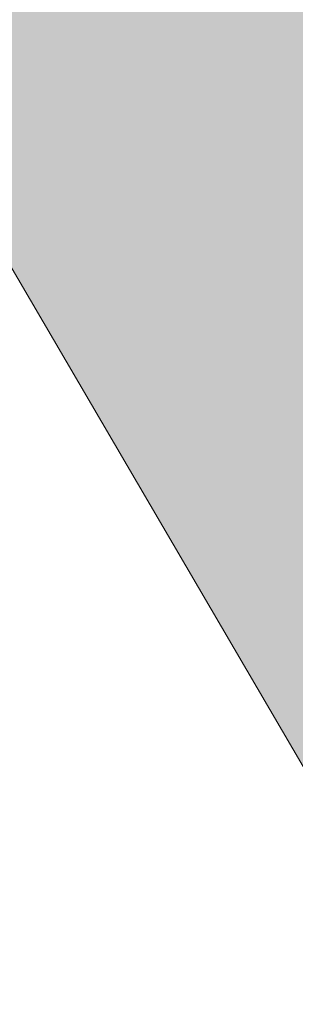
# Model space of a CAD drawing. Units: inches. Extents: x 2091 to 2899, y 967 to 2217.
# Tile 242 of 256: x 2213.361 to 2214.578, y 1131.245 to 1135.592. Entities that reach past the tile are written whole.
import ezdxf

# ---------------------------------------------------------------- set-up
doc = ezdxf.new("R2010")
doc.units = ezdxf.units.IN
doc.layers.add('A-WALL-PATT', color=141, linetype='Continuous', lineweight=13, true_color=0xadddf7)
doc.layers.add('L-PLNT-PATT', color=114, linetype='Continuous', lineweight=13, true_color=0x139b48)
doc.layers.add('L-PLNT-TREE', color=94, linetype='Continuous', lineweight=13)

# ---------------------------------------------------------------- blocks, each defined once
blk = doc.blocks.new('*U25')
blk.add_lwpolyline([(-1139.42368, 1783.79628), (-1216.11644, 1685.47796), (-1117.5111, 1601.2033), (-1051.7759, 1643.3419), (-1126.09884, 1521.20092), (-1072.10606, 1527.49758), (-1079.90386, 1416.93646), (-1259.93906, 1179.83508), (-1479.05978, 1165.78888), (-1577.66258, 1109.60662), (-1742.00312, 927.01364), (-1676.26538, 814.64658), (-1270.89408, 828.69278), (-1194.20386, 772.51052), (-1007.95074, 856.78518), (-876.4778, 575.87134), (-821.70016, 575.87134), (-569.71184, 884.87504)])

msp = doc.modelspace()

# ---------------------------------------------------------------- hatches: boundary and pattern name
at = {"layer": 'A-WALL-PATT'}
h = msp.add_hatch(color=256, dxfattribs=at)
h.dxf.hatch_style = 1
h.paths.add_polyline_path([(2803.1436, 2050.9191), (2203.1436, 2050.9191), (2203.1436, 1090.9191), (2803.1436, 1090.9191)])
h.paths.add_polyline_path([(2635.7989, 1147.5405), (2674.5241, 1147.5405, 0.376086), (2678.5297, 1152.8802), (2678.5297, 1159.5565, 0.333335), (2674.5243, 1163.5618), (2674.5243, 1163.5619), (2674.5243, 1192.9344), (2635.806, 1192.9344), (2597.0876, 1192.9344), (2597.0876, 1163.5618, 0.333335), (2593.0823, 1159.5565), (2593.0823, 1152.8802, 0.376086), (2597.0879, 1147.5405)], flags=0)
h.paths.add_polyline_path([(2436.0104, 1278.2408, 0.000483), (2435.9526, 1278.215, -0.001328), (2435.9356, 1278.1117, -0.001711), (2436.1164, 1278.0408, 0.002185)], flags=0)
h.paths.add_polyline_path([(2794.1436, 1143.4191), (2794.1436, 1347.4191), (2543.3702, 1347.4191), (2543.3702, 1351.9191), (2794.1436, 1351.9191), (2794.1436, 1392.7136), (2793.9474, 1392.7136), (2793.9474, 1473.5369), (2794.1436, 1473.5369), (2794.1436, 1531.9191), (2650.1436, 1531.9191), (2650.1436, 1536.4191), (2794.1436, 1536.4191), (2794.1436, 1692.4191), (2609.3756, 1692.4191), (2609.3756, 1644.4191), (2604.8756, 1644.4191), (2604.8756, 1744.9191), (2609.3756, 1744.9191), (2609.3756, 1696.9191), (2794.1436, 1696.9191), (2794.1436, 1780.9191), (2609.6436, 1780.9191), (2493.8756, 1780.9191), (2493.8756, 1785.4191), (2609.6436, 1785.4191), (2794.1436, 1785.4191), (2794.1436, 1847.9388), (2793.9512, 1847.9388), (2793.9512, 1928.7622), (2794.1436, 1928.7622), (2794.1436, 1941.4191), (2614.1436, 1941.4191), (2614.1436, 1821.4191), (2609.6436, 1821.4191), (2609.6436, 1941.4191), (2392.1436, 1941.4191), (2392.1436, 1819.9191), (2387.6436, 1819.9191), (2387.6436, 1941.4191), (2212.1436, 1941.4191), (2212.1436, 1783.9191), (2392.1436, 1783.9191), (2392.1436, 1780.9191), (2212.1436, 1780.9191), (2212.1436, 1629.4191), (2387.6436, 1629.4191), (2387.6436, 1744.9191), (2392.1436, 1744.9191), (2392.1436, 1627.9191), (2317.1436, 1627.9191), (2317.1436, 1551.4191), (2317.1436, 1536.4191), (2459.3836, 1536.4191), (2459.3836, 1602.3965), (2463.8836, 1602.3965), (2463.8836, 1531.9191), (2456.6436, 1531.9191), (2456.6436, 1529.9191), (2452.1436, 1529.9191), (2452.1436, 1531.9191), (2312.6436, 1531.9191), (2312.6436, 1551.4191), (2306.1436, 1551.4191), (2306.1436, 1555.9191), (2308.1436, 1555.9191), (2308.1436, 1551.4191), (2312.6436, 1551.4191), (2312.6436, 1627.9191), (2212.1436, 1627.9191), (2212.1436, 1555.9191), (2270.1436, 1555.9191), (2270.1436, 1551.4191), (2212.1436, 1551.4191), (2212.1436, 1351.9191), (2272.1436, 1351.9191), (2272.1436, 1347.4191), (2212.1436, 1347.4191), (2212.1436, 1275.4191), (2308.1436, 1275.4191), (2308.1436, 1351.9191), (2452.1436, 1351.9191), (2452.1436, 1493.9191), (2456.6436, 1493.9191), (2456.6436, 1347.4191), (2312.6436, 1347.4191), (2312.6436, 1270.9191), (2212.1436, 1270.9191), (2212.1436, 1099.9191), (2281.2375, 1099.9191), (2282.871, 1110.9138), (2282.0083, 1116.9966), (2278.5577, 1121.4204), (2268.2056, 1128.0562), (2272.0876, 1128.0562), (2273.8129, 1131.927), (2279.4203, 1134.6919), (2285.0278, 1135.2449), (2287.6158, 1137.4568), (2288.0471, 1138.0098), (2289.3411, 1140.7747), (2291.0665, 1139.6687), (2292.3605, 1135.2449), (2295.3798, 1136.9038), (2296.2425, 1135.7979), (2297.1052, 1133.033), (2300.1246, 1138.0098), (2303.1439, 1138.0098), (2304.4379, 1135.7979), (2303.1439, 1133.586), (2306.5946, 1134.6919), (2307.8887, 1133.033), (2310.908, 1135.2449), (2313.9274, 1134.1389), (2315.6269, 1132.4271), (2308.32, 1117.5496), (2290.2038, 1109.8079), (2288.9098, 1103.1721), (2289.2723, 1099.9191), (2434.9182, 1099.9191), (2431.5932, 1124.7881), (2429.9302, 1169.5531), (2430.9272, 1240.5197), (2435.6589, 1238.1861), (2437.1352, 1196.5541), (2438.7982, 1143.9731), (2442.6782, 1111.9981), (2446.5582, 1099.9191), (2794.1436, 1099.9191), (2794.1436, 1138.9191), (2548.0324, 1138.9191), (2548.0324, 1143.4191), (2548.0324, 1148.8191), (2546.6685, 1148.0316), (2528.6857, 1179.1786, 0.256256), (2512.0324, 1148.8191), (2512.0324, 1143.4191), (2512.0324, 1138.9191), (2507.5324, 1138.9191), (2507.5324, 1143.4191), (2507.5324, 1148.8191, 0.256256), (2490.8792, 1179.1786), (2472.8964, 1148.0316), (2471.5324, 1148.8191), (2471.5324, 1143.4191), (2467.0324, 1143.4191), (2467.0324, 1269.9458, 0.039061), (2460.91, 1273.5801), (2467.0324, 1273.5801), (2467.0324, 1286.3254, 0.014511), (2465.2162, 1286.7619), (2467.0324, 1287.0526), (2467.0324, 1323.4191), (2471.5324, 1323.4191), (2471.5324, 1148.8191), (2489.5324, 1179.996), (2490.8964, 1179.2085), (2490.8792, 1179.1786, -0.256256), (2507.5324, 1148.8191), (2507.5324, 1143.4191), (2512.0324, 1143.4191), (2512.0324, 1148.8191, -0.256256), (2528.6857, 1179.1786), (2528.6685, 1179.2085), (2530.0324, 1179.996), (2548.0324, 1148.8191), (2548.0324, 1143.4191)], flags=16)
h.paths.add_polyline_path([(2607.7685, 1200.9451), (2607.7685, 1265.0306), (2597.0876, 1281.052), (2619.7846, 1281.052), (2627.7953, 1337.1269), (2635.7989, 1337.1269), (2643.8167, 1337.1269), (2651.8274, 1281.052), (2674.5243, 1281.052), (2663.8434, 1265.0306), (2663.8434, 1200.9451), (2635.806, 1200.9451)], flags=0)
edge = h.paths.add_edge_path(flags=0)
edge.add_ellipse((13303.8962, 1272.9987), major_axis=(-10595.313, 0), ratio=0.8423038701, start_angle=0.62823722, end_angle=0.6465541, ccw=False)
edge.add_ellipse((2711.7004, 1156.8527), major_axis=(2.2198, 0), ratio=0.842304, start_angle=111.5352, end_angle=180.6282, ccw=False)
edge.add_ellipse((13303.1563, 1272.9987), major_axis=(-10593.0263, 0), ratio=0.8423038695, start_angle=0.52827147, end_angle=0.6465541, ccw=False)
edge.add_line((2710.7646, 1175.3333), (2710.13, 1175.3333))
edge.add_ellipse((2710.13, 1176.5798), major_axis=(1.4798, 0), ratio=0.842304, start_angle=180, end_angle=270, ccw=False)
edge.add_line((2708.6501, 1176.5798), (2708.6501, 1200.7829))
edge.add_ellipse((2710.13, 1200.7829), major_axis=(1.4798, 0), ratio=0.842304, start_angle=90, end_angle=180, ccw=False)
edge.add_line((2710.13, 1202.0294), (2710.4651, 1202.0294))
edge.add_ellipse((13303.1563, 1272.9987), major_axis=(-10593.0263, 0), ratio=0.8423038695, start_angle=-0.09022909, end_angle=0.38386678, ccw=False)
edge.add_ellipse((2710.13, 1290.927), major_axis=(-1.4798, 0), ratio=0.842304, start_angle=0, end_angle=90, ccw=False)
edge.add_line((2708.6501, 1290.927), (2708.6501, 1315.1302))
edge.add_ellipse((2710.13, 1315.1302), major_axis=(-1.4798, 0), ratio=0.842304, start_angle=-90, end_angle=0, ccw=False)
edge.add_line((2710.13, 1316.3767), (2710.7063, 1316.3767))
edge.add_ellipse((3238.4017, 1296.2896), major_axis=(528.234, 0), ratio=0.84230387, start_angle=176.349572, end_angle=177.82005, ccw=False)
edge.add_ellipse((2775.063, 1071.4507), major_axis=(313.3078, 0), ratio=0.84230387, start_angle=102.125966, end_angle=103.780529, ccw=False)
edge.add_ellipse((2775.063, 1078.3057), major_axis=(-305.3029, 0), ratio=0.84230387, start_angle=-79.790461, end_angle=-77.555373, ccw=False)
edge.add_ellipse((2695.1418, 1541.9754), major_axis=(-250.9602, 0), ratio=0.84230387, start_angle=99.256566, end_angle=102.554933)
edge.add_line((2741.4103, 1334.2143), (2747.1325, 1337.3785))
edge.add_ellipse((2747.5386, 1336.8575), major_axis=(-0.7399, 0), ratio=0.842304, start_angle=270, end_angle=307.9331, ccw=False)
edge.add_ellipse((2747.5386, 1336.8575), major_axis=(-0.7399, 0), ratio=0.842304, start_angle=232.0669, end_angle=270, ccw=False)
edge.add_line((2747.9447, 1337.3785), (2753.6669, 1334.2143))
edge.add_ellipse((2799.9355, 1541.9754), major_axis=(250.9602, 0), ratio=0.84230387, start_angle=257.445067, end_angle=260.743434)
edge.add_ellipse((2720.0142, 1078.3057), major_axis=(305.3029, 0), ratio=0.84230387, start_angle=77.555373, end_angle=79.790461, ccw=False)
edge.add_ellipse((2720.0142, 1071.4507), major_axis=(-313.3078, 0), ratio=0.84230387, start_angle=256.219471, end_angle=257.874034, ccw=False)
edge.add_ellipse((2256.6755, 1296.2896), major_axis=(-528.234, 0), ratio=0.84230387, start_angle=182.17995, end_angle=183.650428, ccw=False)
edge.add_line((2784.3709, 1316.3767), (2784.9472, 1316.3767))
edge.add_ellipse((2784.9472, 1315.1302), major_axis=(1.4798, 0), ratio=0.842304, start_angle=0, end_angle=90, ccw=False)
edge.add_line((2786.4271, 1315.1302), (2786.4271, 1290.927))
edge.add_ellipse((2784.9472, 1290.927), major_axis=(1.4798, 0), ratio=0.842304, start_angle=270, end_angle=360, ccw=False)
edge.add_ellipse((-7808.0791, 1272.9987), major_axis=(10593.0263, 0), ratio=0.8423038695, start_angle=-0.38386678, end_angle=0.09022909, ccw=False)
edge.add_line((2784.6122, 1202.0294), (2784.9472, 1202.0294))
edge.add_ellipse((2784.9472, 1200.7829), major_axis=(1.4798, 0), ratio=0.842304, start_angle=0, end_angle=90, ccw=False)
edge.add_line((2786.4271, 1200.7829), (2786.4271, 1176.5798))
edge.add_ellipse((2784.9472, 1176.5798), major_axis=(-1.4798, 0), ratio=0.842304, start_angle=90, end_angle=180, ccw=False)
edge.add_line((2784.9472, 1175.3333), (2784.3126, 1175.3333))
edge.add_ellipse((-7808.0791, 1272.9987), major_axis=(10593.0263, 0), ratio=0.8423038695, start_angle=-0.6186432, end_angle=-0.52827147, ccw=False)
edge.add_ellipse((2783.3768, 1156.8527), major_axis=(-2.2198, 0), ratio=0.842304, start_angle=179.3718, end_angle=248.4648, ccw=False)
edge.add_ellipse((-7808.819, 1272.9987), major_axis=(-10595.313, 0), ratio=0.8423038658, start_angle=179.35344592, end_angle=179.3717628, ccw=False)
edge.add_ellipse((2780.2973, 1153.5008), major_axis=(-5.2464, 0), ratio=0.842304, start_angle=90, end_angle=179.3534, ccw=False)
edge.add_line((2780.2973, 1149.0817), (2714.7799, 1149.0817))
edge.add_ellipse((2714.7799, 1153.5008), major_axis=(5.2464, 0), ratio=0.842304, start_angle=180.6466, end_angle=270, ccw=False)
edge = h.paths.add_edge_path(flags=0)
edge.add_line((2718.1874, 1151.0078), (2718.1874, 1170.4724))
edge.add_ellipse((2721.1471, 1170.4724), major_axis=(-2.9597, 0), ratio=0.842304, start_angle=-90, end_angle=0, ccw=False)
edge.add_line((2721.1471, 1172.9653), (2773.9302, 1172.9653))
edge.add_ellipse((2773.9302, 1170.4724), major_axis=(-2.9597, 0), ratio=0.842304, start_angle=180, end_angle=270, ccw=False)
edge.add_line((2776.8899, 1170.4724), (2776.8899, 1151.0078))
edge.add_line((2776.8899, 1151.0078), (2718.1874, 1151.0078))
edge = h.paths.add_edge_path(flags=0)
edge.add_line((2718.1874, 1180.2342), (2718.1874, 1199.0578))
edge.add_ellipse((2747.5386, 1320.3986), major_axis=(147.0179, 0), ratio=0.84230387, start_angle=256.401865, end_angle=283.598135)
edge.add_line((2776.8899, 1199.0578), (2776.8899, 1180.2342))
edge.add_ellipse((2747.5386, 1301.575), major_axis=(147.0179, 0), ratio=0.84230387, start_angle=256.401865, end_angle=283.598135, ccw=False)
edge = h.paths.add_edge_path(flags=0)
edge.add_ellipse((13303.1563, 1272.9987), major_axis=(-10591.5465, 0), ratio=0.8423038696, start_angle=0.05559431, end_angle=0.37776419, ccw=False)
edge.add_line((2711.6169, 1262.7217), (2715.6674, 1249.4954))
edge.add_ellipse((6413.892, 1241.6919), major_axis=(-3698.2362, 0), ratio=0.84230387, start_angle=-0.1208974, end_angle=0.3640763)
edge.add_line((2715.761, 1218.1925), (2711.9343, 1203.1674))
edge = h.paths.add_edge_path(flags=0)
edge.add_line((2718.1874, 1251.0746), (2716.0025, 1267.4504))
edge.add_ellipse((2742.1512, 1202.1895), major_axis=(81.7726, 0), ratio=0.8423039, start_angle=94.277421, end_angle=111.834954, ccw=False)
edge.add_line((2737.0097, 1270.9306), (2758.0675, 1270.9306))
edge.add_ellipse((2752.9261, 1202.1895), major_axis=(81.7726, 0), ratio=0.8423039, start_angle=68.165046, end_angle=85.722579, ccw=False)
edge.add_line((2779.0747, 1267.4504), (2776.8899, 1251.0746))
edge.add_ellipse((2750.3381, 1187.8854), major_axis=(79.5797, 0), ratio=0.8423039, start_angle=67.208085, end_angle=85.12993)
edge.add_line((2756.0347, 1254.7437), (2739.0426, 1254.7437))
edge.add_ellipse((2744.7392, 1187.8854), major_axis=(79.5797, 0), ratio=0.8423039, start_angle=94.87007, end_angle=112.791915)
edge = h.paths.add_edge_path(flags=0)
edge.add_line((2783.1429, 1203.1674), (2779.3162, 1218.1925))
edge.add_ellipse((-918.8147, 1241.6919), major_axis=(3698.2362, 0), ratio=0.84230387, start_angle=-0.3640763, end_angle=0.1208974)
edge.add_line((2779.4098, 1249.4954), (2783.4604, 1262.7217))
edge.add_ellipse((-7808.0791, 1272.9987), major_axis=(-10591.5465, 0), ratio=0.8423038695, start_angle=179.62223581, end_angle=179.94440569, ccw=False)
edge = h.paths.add_edge_path(flags=0)
edge.add_ellipse((2734.2009, 1286.6904), major_axis=(-0.3566, 6.3401), ratio=0.603834, start_angle=89.00201, end_angle=253.65741, ccw=False)
edge.add_line((2730.369, 1286.5418), (2730.369, 1301.352))
edge.add_line((2730.369, 1301.352), (2735.9133, 1305.2148))
edge.add_ellipse((2736.3849, 1304.7346), major_axis=(0.7399, 0), ratio=0.842304, start_angle=90, end_angle=134.4802, ccw=False)
edge.add_line((2736.3849, 1305.3578), (2738.0328, 1305.3578))
edge.add_line((2738.0328, 1305.3578), (2738.0328, 1307.7079))
edge.add_ellipse((2794.2016, 1307.7079), major_axis=(56.1689, 0), ratio=0.8423039, start_angle=150.56143, end_angle=180, ccw=False)
edge.add_ellipse((2700.8756, 1307.7079), major_axis=(-56.1689, 0), ratio=0.8423039, start_angle=180, end_angle=209.43857, ccw=False)
edge.add_line((2757.0444, 1307.7079), (2757.0444, 1305.3578))
edge.add_line((2757.0444, 1305.3578), (2758.6923, 1305.3578))
edge.add_ellipse((2758.6923, 1304.7346), major_axis=(-0.7399, 0), ratio=0.842304, start_angle=225.5198, end_angle=270, ccw=False)
edge.add_line((2759.1639, 1305.2148), (2764.7082, 1301.352))
edge.add_line((2764.7082, 1301.352), (2764.7082, 1286.5418))
edge.add_ellipse((2760.8763, 1286.6904), major_axis=(0.3566, 6.3401), ratio=0.603834, start_angle=106.34259, end_angle=270.99799, ccw=False)
edge.add_line((2757.0444, 1285.7971), (2757.0444, 1307.7079))
edge.add_ellipse((2700.8756, 1307.7079), major_axis=(-56.1689, 0), ratio=0.8423039, start_angle=180, end_angle=209.43857)
edge.add_ellipse((2794.2016, 1307.7079), major_axis=(56.1689, 0), ratio=0.8423039, start_angle=150.56143, end_angle=180)
edge.add_line((2738.0328, 1307.7079), (2738.0328, 1285.7971))
h.paths.add_polyline_path([(2417.8123, 1104.4497), (2413.4923, 1102.5297), (2410.6123, 1103.9697), (2409.1723, 1106.3697), (2407.2523, 1107.3297), (2406.2923, 1109.7297), (2405.3323, 1114.0497), (2405.3323, 1117.8897), (2406.2923, 1120.1297), (2407.2523, 1119.8097), (2408.8483, 1118.3277), (2410.1739, 1119.4242), (2410.2113, 1120.4057), (2411.0407, 1121.4191), (2410.6993, 1119.8587), (2410.1739, 1119.4242), (2410.0885, 1117.1761), (2411.1328, 1116.2063), (2413.9723, 1119.3297), (2416.8523, 1120.7697), (2416.8697, 1120.7988), (2417.0351, 1119.4051), (2417.8962, 1118.1434), (2418.2923, 1118.3697), (2419.5444, 1120.0393), (2419.3609, 1118.3875), (2419.0321, 1119.3562), (2418.3989, 1118.5119), (2419.2523, 1114.5297), (2418.7941, 1107.1988)], flags=0)
h.paths.add_polyline_path([(2508.8702, 1347.4191), (2508.3702, 1347.4191), (2508.3702, 1351.9191), (2508.8702, 1351.9191)], flags=0)
h.paths.add_polyline_path([(2473.3702, 1347.4191), (2472.3702, 1347.4191), (2467.8702, 1347.4191), (2467.8702, 1455.4191), (2472.3702, 1455.4191), (2472.3702, 1352.4191), (2473.3702, 1352.4191)], flags=0)
h.paths.add_polyline_path([(2352.1062, 1217.4462), (2349.2262, 1218.8862), (2347.7862, 1221.2862), (2345.8662, 1222.2462), (2344.9062, 1224.6462), (2343.9462, 1228.9662), (2343.9462, 1232.8062), (2344.9062, 1235.0462), (2345.8662, 1234.7262), (2347.4623, 1233.2442), (2348.7879, 1234.3407), (2348.8252, 1235.3222), (2349.6547, 1236.3355), (2349.3132, 1234.7752), (2348.7879, 1234.3407), (2348.7024, 1232.0926), (2349.7468, 1231.1228), (2352.5862, 1234.2462), (2355.4662, 1235.6862), (2355.4837, 1235.7153), (2355.649, 1234.3216), (2356.5102, 1233.0599), (2356.9062, 1233.2862), (2358.1584, 1234.9558), (2357.9749, 1233.304), (2357.6461, 1234.2726), (2357.0129, 1233.4284), (2357.8662, 1229.4462), (2357.4081, 1222.1153), (2356.4262, 1219.3662)], flags=0)
h.paths.add_polyline_path([(2348.2968, 1112.2244), (2347.0138, 1112.3104), (2345.5298, 1114.1274), (2345.7318, 1115.8584), (2346.8118, 1116.9824), (2346.8118, 1114.6464), (2345.8668, 1114.2144), (2346.8798, 1114.3004)], flags=0)
h.paths.add_polyline_path([(2347.0138, 1110.9264), (2346.2718, 1110.4934), (2346.6098, 1111.1864)], flags=0)
h.paths.add_polyline_path([(2345.8668, 1118.1944), (2345.5298, 1117.3294), (2343.7078, 1118.0214), (2344.3828, 1118.6264)], flags=0)
h.paths.add_polyline_path([(2346.6768, 1109.2824), (2346.0698, 1108.0714), (2345.8668, 1110.0614)], flags=0)
h.paths.add_polyline_path([(2345.0568, 1119.7514), (2343.6398, 1119.7514), (2343.9778, 1121.1354)], flags=0)
h.paths.add_polyline_path([(2345.2598, 1116.5504), (2345.1248, 1115.8584), (2344.9218, 1115.6854), (2344.7198, 1116.3774)], flags=0)
h.paths.add_polyline_path([(2345.6648, 1112.3104), (2345.4618, 1111.5324), (2344.0448, 1111.9644), (2344.6518, 1112.5704)], flags=0)
h.paths.add_polyline_path([(2345.1918, 1113.3494), (2344.4498, 1113.8684), (2344.7198, 1114.3874)], flags=0)
h.paths.add_polyline_path([(2344.6518, 1116.8094), (2344.1798, 1115.6854), (2344.6518, 1115.3394), (2343.9098, 1114.9064), (2343.0328, 1115.9444), (2343.6398, 1116.4634)], flags=0)
h.paths.add_polyline_path([(2345.8668, 1106.6864), (2344.9898, 1105.5624), (2344.5168, 1106.6004)], flags=0)
h.paths.add_polyline_path([(2344.8548, 1110.0614), (2344.5168, 1109.2824), (2344.1128, 1109.7154)], flags=0)
h.paths.add_polyline_path([(2344.0448, 1113.5224), (2343.4378, 1113.0894), (2342.7628, 1113.9544)], flags=0)
h.paths.add_polyline_path([(2344.3148, 1111.0124), (2342.9648, 1110.3204), (2342.9648, 1111.0994)], flags=0)
h.paths.add_polyline_path([(2345.1248, 1104.6974), (2344.5848, 1103.7454), (2344.4498, 1104.2644)], flags=0)
h.paths.add_polyline_path([(2342.8298, 1121.2224), (2341.7498, 1120.5304), (2340.5358, 1121.0494), (2340.1308, 1121.8284), (2340.6708, 1122.9524), (2341.1428, 1121.8284), (2341.6148, 1122.0014)], flags=0)
h.paths.add_polyline_path([(2342.9648, 1119.7514), (2343.0328, 1118.4534), (2342.0878, 1118.0214), (2342.0198, 1119.4914)], flags=0)
h.paths.add_polyline_path([(2342.6948, 1116.8964), (2341.9528, 1116.6364), (2342.0198, 1117.3294)], flags=0)
h.paths.add_polyline_path([(2343.0328, 1112.2244), (2342.0198, 1111.7914), (2341.5478, 1112.2244), (2342.3578, 1113.3494)], flags=0)
h.paths.add_polyline_path([(2343.7748, 1104.4374), (2342.6278, 1102.8804), (2342.6948, 1104.6104), (2343.4378, 1105.1294)], flags=0)
h.paths.add_polyline_path([(2342.0198, 1115.0794), (2340.8058, 1115.5124), (2340.9408, 1116.3774)], flags=0)
h.paths.add_polyline_path([(2341.4808, 1120.0974), (2341.4808, 1119.4054), (2341.0758, 1119.5784), (2341.1428, 1120.0974)], flags=0)
h.paths.add_polyline_path([(2341.8178, 1114.4734), (2340.9408, 1113.0894), (2340.8058, 1114.5604)], flags=0)
h.paths.add_polyline_path([(2341.1428, 1118.5404), (2340.9408, 1116.9824), (2339.0508, 1117.6754), (2339.0508, 1118.6264)], flags=0)
h.paths.add_polyline_path([(2342.6948, 1101.6684), (2341.9528, 1101.8414), (2342.5598, 1102.3614)], flags=0)
h.paths.add_polyline_path([(2340.3328, 1119.6654), (2338.4438, 1119.5784), (2337.9038, 1120.3574), (2339.6578, 1120.6164)], flags=0)
h.paths.add_polyline_path([(2340.3328, 1115.3394), (2340.0628, 1113.6954), (2339.3878, 1115.3394)], flags=0)
h.paths.add_polyline_path([(2341.8178, 1103.8314), (2341.5478, 1102.8804), (2341.1428, 1103.6584)], flags=0)
h.paths.add_polyline_path([(2339.0508, 1122.8664), (2337.2958, 1121.8284), (2337.0938, 1123.1254), (2337.7688, 1123.8184)], flags=0)
h.paths.add_polyline_path([(2339.1178, 1121.7414), (2338.8478, 1121.2224), (2338.1738, 1121.0494), (2338.3758, 1121.5684)], flags=0)
h.paths.add_polyline_path([(2339.1858, 1119.3194), (2338.6458, 1118.7134), (2338.2408, 1118.1074), (2338.2408, 1118.8864)], flags=0)
h.paths.add_polyline_path([(2341.1428, 1101.9284), (2340.6028, 1101.2364), (2340.0628, 1101.8414), (2340.6028, 1102.3614)], flags=0)
h.paths.add_polyline_path([(2337.6338, 1117.7614), (2336.6208, 1118.2804), (2337.2958, 1118.9724)], flags=0)
h.paths.add_polyline_path([(2336.8238, 1119.5784), (2334.7988, 1118.9724), (2335.2038, 1120.3574), (2336.5538, 1120.8764)], flags=0)
h.paths.add_polyline_path([(2339.1178, 1100.4574), (2337.3638, 1100.5434), (2336.7558, 1101.2364)], flags=0)
h.paths.add_polyline_path([(2336.3508, 1122.4334), (2336.0138, 1121.9144), (2334.9338, 1122.4334), (2334.5288, 1123.4714), (2335.7438, 1122.7794)], flags=0)
h.paths.add_polyline_path([(2334.7318, 1120.8764), (2334.2588, 1120.3574), (2334.0568, 1120.7894), (2334.5968, 1121.3084)], flags=0)
h.paths.add_polyline_path([(2334.4618, 1122.1744), (2332.5718, 1121.3084), (2331.3568, 1122.1744), (2332.0998, 1122.8664)], flags=0)
h.paths.add_polyline_path([(2334.2588, 1118.5404), (2333.3818, 1118.4534), (2333.6518, 1119.3194)], flags=0)
h.paths.add_polyline_path([(2335.5418, 1102.2744), (2334.1918, 1102.6204), (2335.2718, 1103.3124)], flags=0)
h.paths.add_polyline_path([(2332.7068, 1119.6654), (2331.6948, 1120.4434), (2332.5048, 1120.7894)], flags=0)
h.paths.add_polyline_path([(2334.7318, 1101.1494), (2333.5168, 1101.5824), (2333.9888, 1101.7554)], flags=0)
h.paths.add_polyline_path([(2332.6398, 1116.6364), (2331.0868, 1116.2904), (2331.9648, 1118.1944)], flags=0)
h.paths.add_polyline_path([(2330.7498, 1121.5684), (2330.2768, 1120.2704), (2328.5228, 1119.3194), (2328.9948, 1121.0494)], flags=0)
h.paths.add_polyline_path([(2330.7498, 1118.6264), (2330.0078, 1117.5024), (2329.8728, 1118.0214)], flags=0)
h.paths.add_polyline_path([(2332.0998, 1102.3614), (2330.5468, 1102.0144), (2331.6948, 1102.9664)], flags=0)
h.paths.add_polyline_path([(2329.5348, 1113.6084), (2329.0628, 1112.3104), (2328.5898, 1113.3494)], flags=0)
h.paths.add_polyline_path([(2328.3878, 1117.8484), (2327.5098, 1116.5504), (2327.1728, 1117.7614)], flags=0)
h.paths.add_polyline_path([(2329.7378, 1106.5134), (2329.5348, 1105.3024), (2328.2528, 1106.0814)], flags=0)
h.paths.add_polyline_path([(2328.6578, 1114.3874), (2328.0498, 1114.1274), (2328.3198, 1114.9064)], flags=0)
h.paths.add_polyline_path([(2328.3198, 1112.2244), (2327.1058, 1112.1374), (2326.7008, 1112.6564)], flags=0)
h.paths.add_polyline_path([(2326.9028, 1115.2524), (2326.7008, 1114.1274), (2325.2158, 1113.6084), (2326.0928, 1115.3394)], flags=0)
h.paths.add_polyline_path([(2326.6328, 1108.3304), (2326.0928, 1107.3794), (2325.8908, 1108.5034), (2326.4978, 1109.1094)], flags=0)
h.paths.add_polyline_path([(2615.1436, 1531.9191), (2609.6436, 1531.9191), (2609.6436, 1620.4191), (2614.1436, 1620.4191), (2614.1436, 1536.4191), (2615.1436, 1536.4191)], flags=0)
h.paths.add_polyline_path([(2545.1436, 1563.4191), (2464.1436, 1563.4191), (2464.1436, 1632.4191), (2509.1436, 1632.4191), (2509.1436, 1627.9191), (2509.1436, 1603.9191), (2468.6436, 1603.9191), (2468.6436, 1567.9191), (2540.6436, 1567.9191), (2540.6436, 1591.9191), (2545.1436, 1591.9191)], flags=0)
h.paths.add_polyline_path([(2388.969, 1549.9857), (2357.4342, 1549.9857), (2357.4342, 1623.3608), (2399.3628, 1623.3608), (2435.6895, 1623.3608), (2435.5925, 1602.5593), (2435.5925, 1602.3965), (2388.969, 1602.3965)], flags=0)
h.paths.add_polyline_path([(2388.8806, 1555.8092), (2374.9044, 1555.8092), (2374.9044, 1600.5716), (2374.9044, 1615.4576), (2406.3509, 1615.4576), (2406.3509, 1618.9394), (2412.1743, 1615.4576), (2406.3509, 1611.9759), (2406.3509, 1615.4576), (2388.8806, 1615.4576)], flags=0)
h.paths.add_polyline_path([(2568.8756, 1644.4191), (2453.3756, 1644.4191), (2453.3756, 1785.4191), (2457.8756, 1785.4191), (2457.8756, 1648.9191), (2568.8756, 1648.9191)], flags=0)
h.paths.add_polyline_path([(2212.1436, 1945.9191), (2212.1436, 2041.9191), (2794.1436, 2041.9191), (2794.1436, 1945.9191)], flags=16)
h.paths.add_polyline_path([(2271.0827, 1964.3172), (2776.853, 1964.3172), (2776.853, 2037.1696), (2271.0827, 2037.1696)], flags=8)
h.paths.add_polyline_path([(2380.6493, 1536.8241), (2461.0408, 1536.8241), (2461.0408, 1554.6526), (2380.6493, 1554.6526)], flags=8)
h.paths.add_polyline_path([(2240.7557, 1609.7255), (2309.1858, 1609.7255), (2309.1858, 1617.6982), (2240.7557, 1617.6982)], flags=8)
h.paths.add_polyline_path([(2212.6773, 1313.5041), (2282.5915, 1313.5041), (2282.5915, 1322.7452), (2212.6773, 1322.7452)], flags=8)
h.paths.add_polyline_path([(2457.112, 1114.7786), (2558.4816, 1114.7786), (2558.4816, 1142.2197), (2457.112, 1142.2197)], flags=8)
h.paths.add_polyline_path([(2473.4423, 1273.0101), (2604.6412, 1273.0101), (2604.6412, 1318.3469), (2473.4423, 1318.3469)], flags=8)
h.paths.add_polyline_path([(2638.8763, 1626.9774), (2684.2504, 1627.9767), (2684.0385, 1637.5975), (2638.6644, 1636.5982)], flags=8)
h.paths.add_polyline_path([(2537.5906, 1453.7934), (2628.3895, 1453.7934), (2628.3895, 1475.3448), (2537.5906, 1475.3448)], flags=8)
h.paths.add_polyline_path([(2504.1376, 1714.6324), (2554.6472, 1714.6324), (2554.6472, 1730.2377), (2504.1376, 1730.2377)], flags=8)
h.paths.add_polyline_path([(2487.5012, 1575.6519), (2535.0971, 1575.6519), (2535.0971, 1598.3776), (2487.5012, 1598.3776)], flags=8)
h.paths.add_polyline_path([(2709.0994, 1735.7103), (2740.0166, 1735.7103), (2740.0166, 1749.9376), (2709.0994, 1749.9376)], flags=8)
h.paths.add_polyline_path([(2442.4384, 1792.1717), (2564.7288, 1792.1717), (2564.7288, 1842.0002), (2442.4384, 1842.0002)], flags=8)
h.paths.add_polyline_path([(2655.8158, 1809.6441), (2789.5201, 1806.6938), (2790.085, 1832.2916), (2656.3806, 1835.2419)], flags=8)
h.paths.add_polyline_path([(2234.8427, 1797.7201), (2368.5929, 1794.7689), (2369.1607, 1820.5041), (2235.4106, 1823.4554)], flags=8)
h.paths.add_polyline_path([(2245.1385, 1644.0063), (2398.4277, 1640.6239), (2398.9948, 1666.3248), (2245.7056, 1669.7073)], flags=8)
h.paths.add_polyline_path([(2306.1428, 1431.1685), (2413.7683, 1428.7937), (2414.3331, 1454.3915), (2306.7077, 1456.7664)], flags=8)
h.paths.add_polyline_path([(2306.8346, 1458.2331), (2393.3805, 1456.3234), (2393.9328, 1481.3544), (2307.3869, 1483.2641)], flags=8)
at = {"layer": 'L-PLNT-PATT'}
h = msp.add_hatch(color=256, dxfattribs=at)
h.dxf.hatch_style = 1
h.paths.add_polyline_path([(2333.3376, 1165.6587), (2329.0242, 1166.2116), (2331.6122, 1168.4235), (2335.0629, 1177.2712), (2328.1615, 1184.4599), (2319.5348, 1187.2248), (2323.4168, 1193.3076), (2319.9661, 1203.8142), (2317.8094, 1203.8142), (2313.496, 1213.2148), (2310.908, 1212.6618), (2307.8887, 1212.6618), (2305.7319, 1217.0857), (2307.0259, 1223.1684), (2310.4767, 1223.1684), (2304.0066, 1230.9101), (2303.1363, 1237.0465), (2299.6932, 1240.8637), (2296.6739, 1237.5459), (2294.9485, 1238.6518), (2294.5171, 1241.4166), (2292.3605, 1242.5227), (2289.3411, 1239.7577), (2285.8904, 1240.3107), (2283.3024, 1235.3339), (2283.3024, 1230.9101), (2286.7531, 1229.2512), (2284.165, 1227.5922), (2281.577, 1229.8042), (2274.2442, 1222.6154), (2274.2442, 1220.9565), (2271.2249, 1219.2976), (2272.0876, 1217.6386), (2274.2442, 1214.3208), (2270.3622, 1211.5559), (2266.4801, 1214.3208), (2264.3235, 1213.7678), (2263.4608, 1211.5559), (2266.4801, 1211.0029), (2266.9115, 1206.5791), (2263.5392, 1207.132), (2259.5788, 1203.2612), (2263.8921, 1202.7082), (2262.1668, 1197.1784), (2258.2848, 1196.6254), (2253.9714, 1193.8606), (2248.7953, 1191.0957), (2248.364, 1193.3076), (2244.4819, 1185.0129), (2251.3833, 1186.6718), (2255.6967, 1183.9069), (2254.4027, 1177.2712), (2246.6387, 1174.5063), (2243.1879, 1176.7182), (2241.8939, 1173.4003), (2238.8746, 1172.8474), (2236.2865, 1169.5295), (2233.2671, 1165.6587), (2237.1492, 1162.3408), (2239.7372, 1163.9998), (2236.8111, 1159.1911), (2238.9368, 1159.439), (2238.6298, 1155.0862), (2231.5418, 1145.7515), (2222.915, 1145.1985), (2219.033, 1142.9866), (2212.5629, 1135.7979), (2215.151, 1131.374), (2231.1105, 1131.927), (2234.1298, 1129.7151), (2241.4626, 1133.033), (2246.6387, 1121.9734), (2248.7953, 1121.9734), (2258.7161, 1134.1389), (2261.7355, 1135.7979), (2263.8921, 1133.033), (2263.8921, 1129.1621), (2267.3429, 1128.0562), (2272.0876, 1128.0562), (2273.8129, 1131.927), (2279.4203, 1134.6919), (2285.0278, 1135.2449), (2287.6158, 1137.4568), (2288.0471, 1138.0098), (2289.3411, 1140.7747), (2291.0665, 1139.6687), (2292.3605, 1135.2449), (2295.3798, 1136.9038), (2296.2425, 1135.7979), (2297.1052, 1133.033), (2300.1246, 1138.0098), (2303.1439, 1138.0098), (2304.4379, 1135.7979), (2303.1439, 1133.586), (2306.5946, 1134.6919), (2307.8887, 1133.033), (2310.908, 1135.2449), (2313.9274, 1134.1389), (2319.9661, 1128.0562), (2322.5541, 1126.9502), (2324.7108, 1124.7383), (2342.827, 1126.3972), (2346.2777, 1123.0794), (2348.8658, 1124.1853), (2341.9643, 1133.033), (2341.533, 1136.3508), (2343.6897, 1139.6687), (2339.8077, 1150.1753), (2337.651, 1150.1753)])
h.paths.add_polyline_path([(2339.6578, 1120.6164), (2337.9038, 1120.3574), (2338.4438, 1119.5784), (2340.3328, 1119.6654)])
h.paths.add_polyline_path([(2341.1428, 1118.5404), (2339.0508, 1118.6264), (2339.0508, 1117.6754), (2340.9408, 1116.9824)])
h.paths.add_polyline_path([(2336.5538, 1120.8764), (2335.2038, 1120.3574), (2334.7988, 1118.9724), (2336.8238, 1119.5784)])
h.paths.add_polyline_path([(2337.2958, 1118.9724), (2336.6208, 1118.2804), (2337.6338, 1117.7614)])
h.paths.add_polyline_path([(2338.6458, 1118.7134), (2339.1858, 1119.3194), (2338.2408, 1118.8864), (2338.2408, 1118.1074)])
h.paths.add_polyline_path([(2339.0508, 1122.8664), (2337.7688, 1123.8184), (2337.0938, 1123.1254), (2337.2958, 1121.8284)])
h.paths.add_polyline_path([(2341.6148, 1122.0014), (2341.1428, 1121.8284), (2340.6708, 1122.9524), (2340.1308, 1121.8284), (2340.5358, 1121.0494), (2341.7498, 1120.5304), (2342.8298, 1121.2224)])
h.paths.add_polyline_path([(2342.9648, 1119.7514), (2342.0198, 1119.4914), (2342.0878, 1118.0214), (2343.0328, 1118.4534)])
h.paths.add_polyline_path([(2345.8668, 1118.1944), (2344.3828, 1118.6264), (2343.7078, 1118.0214), (2345.5298, 1117.3294)])
h.paths.add_polyline_path([(2344.6518, 1116.8094), (2343.6398, 1116.4634), (2343.0328, 1115.9444), (2343.9098, 1114.9064), (2344.6518, 1115.3394), (2344.1798, 1115.6854)])
h.paths.add_polyline_path([(2346.8118, 1116.9824), (2345.7318, 1115.8584), (2345.5298, 1114.1274), (2347.0138, 1112.3104), (2348.2968, 1112.2244), (2346.8798, 1114.3004), (2345.8668, 1114.2144), (2346.8118, 1114.6464)])
h.paths.add_polyline_path([(2345.2598, 1116.5504), (2344.7198, 1116.3774), (2344.9218, 1115.6854), (2345.1248, 1115.8584)])
h.paths.add_polyline_path([(2342.6948, 1116.8964), (2342.0198, 1117.3294), (2341.9528, 1116.6364)])
h.paths.add_polyline_path([(2341.4808, 1120.0974), (2341.1428, 1120.0974), (2341.0758, 1119.5784), (2341.4808, 1119.4054)])
h.paths.add_polyline_path([(2343.9778, 1121.1354), (2343.6398, 1119.7514), (2345.0568, 1119.7514)])
h.paths.add_polyline_path([(2339.1178, 1121.7414), (2338.3758, 1121.5684), (2338.1738, 1121.0494), (2338.8478, 1121.2224)])
h.paths.add_polyline_path([(2336.3508, 1122.4334), (2335.7438, 1122.7794), (2334.5288, 1123.4714), (2334.9338, 1122.4334), (2336.0138, 1121.9144)])
h.paths.add_polyline_path([(2334.4618, 1122.1744), (2332.0998, 1122.8664), (2331.3568, 1122.1744), (2332.5718, 1121.3084)])
h.paths.add_polyline_path([(2334.5968, 1121.3084), (2334.0568, 1120.7894), (2334.2588, 1120.3574), (2334.7318, 1120.8764)])
h.paths.add_polyline_path([(2332.5048, 1120.7894), (2331.6948, 1120.4434), (2332.7068, 1119.6654)])
h.paths.add_polyline_path([(2333.6518, 1119.3194), (2333.3818, 1118.4534), (2334.2588, 1118.5404)])
h.paths.add_polyline_path([(2331.9648, 1118.1944), (2331.0868, 1116.2904), (2332.6398, 1116.6364)])
h.paths.add_polyline_path([(2330.7498, 1121.5684), (2328.9948, 1121.0494), (2328.5228, 1119.3194), (2330.2768, 1120.2704)])
h.paths.add_polyline_path([(2330.7498, 1118.6264), (2329.8728, 1118.0214), (2330.0078, 1117.5024)])
h.paths.add_polyline_path([(2328.3878, 1117.8484), (2327.1728, 1117.7614), (2327.5098, 1116.5504)])
h.paths.add_polyline_path([(2326.9028, 1115.2524), (2326.0928, 1115.3394), (2325.2158, 1113.6084), (2326.7008, 1114.1274)])
h.paths.add_polyline_path([(2328.6578, 1114.3874), (2328.3198, 1114.9064), (2328.0498, 1114.1274)])
h.paths.add_polyline_path([(2326.7008, 1112.6564), (2327.1058, 1112.1374), (2328.3198, 1112.2244)])
h.paths.add_polyline_path([(2329.5348, 1113.6084), (2328.5898, 1113.3494), (2329.0628, 1112.3104)])
h.paths.add_polyline_path([(2340.3328, 1115.3394), (2339.3878, 1115.3394), (2340.0628, 1113.6954)])
h.paths.add_polyline_path([(2340.9408, 1116.3774), (2340.8058, 1115.5124), (2342.0198, 1115.0794)])
h.paths.add_polyline_path([(2341.8178, 1114.4734), (2340.8058, 1114.5604), (2340.9408, 1113.0894)])
h.paths.add_polyline_path([(2343.0328, 1112.2244), (2342.3578, 1113.3494), (2341.5478, 1112.2244), (2342.0198, 1111.7914)])
h.paths.add_polyline_path([(2342.7628, 1113.9544), (2343.4378, 1113.0894), (2344.0448, 1113.5224)])
h.paths.add_polyline_path([(2344.7198, 1114.3874), (2344.4498, 1113.8684), (2345.1918, 1113.3494)])
h.paths.add_polyline_path([(2345.6648, 1112.3104), (2344.6518, 1112.5704), (2344.0448, 1111.9644), (2345.4618, 1111.5324)])
h.paths.add_polyline_path([(2344.3148, 1111.0124), (2342.9648, 1111.0994), (2342.9648, 1110.3204)])
h.paths.add_polyline_path([(2344.8548, 1110.0614), (2344.1128, 1109.7154), (2344.5168, 1109.2824)])
h.paths.add_polyline_path([(2346.6768, 1109.2824), (2345.8668, 1110.0614), (2346.0698, 1108.0714)])
h.paths.add_polyline_path([(2347.0138, 1110.9264), (2346.6098, 1111.1864), (2346.2718, 1110.4934)])
h.paths.add_polyline_path([(2345.8668, 1106.6864), (2344.5168, 1106.6004), (2344.9898, 1105.5624)])
h.paths.add_polyline_path([(2345.1248, 1104.6974), (2344.4498, 1104.2644), (2344.5848, 1103.7454)])
h.paths.add_polyline_path([(2343.7748, 1104.4374), (2343.4378, 1105.1294), (2342.6948, 1104.6104), (2342.6278, 1102.8804)])
h.paths.add_polyline_path([(2341.8178, 1103.8314), (2341.1428, 1103.6584), (2341.5478, 1102.8804)])
h.paths.add_polyline_path([(2342.5598, 1102.3614), (2341.9528, 1101.8414), (2342.6948, 1101.6684)])
h.paths.add_polyline_path([(2341.1428, 1101.9284), (2340.6028, 1102.3614), (2340.0628, 1101.8414), (2340.6028, 1101.2364)])
h.paths.add_polyline_path([(2336.7558, 1101.2364), (2337.3638, 1100.5434), (2339.1178, 1100.4574)])
h.paths.add_polyline_path([(2335.2718, 1103.3124), (2334.1918, 1102.6204), (2335.5418, 1102.2744)])
h.paths.add_polyline_path([(2333.9888, 1101.7554), (2333.5168, 1101.5824), (2334.7318, 1101.1494)])
h.paths.add_polyline_path([(2331.6948, 1102.9664), (2330.5468, 1102.0144), (2332.0998, 1102.3614)])
h.paths.add_polyline_path([(2329.7378, 1106.5134), (2328.2528, 1106.0814), (2329.5348, 1105.3024)])
h.paths.add_polyline_path([(2326.6328, 1108.3304), (2326.4978, 1109.1094), (2325.8908, 1108.5034), (2326.0928, 1107.3794)])
h.paths.add_polyline_path([(2240.5961, 1257.8142), (2239.5841, 1257.4682), (2238.9771, 1256.9492), (2239.8541, 1255.9112), (2240.5961, 1256.3442), (2240.1241, 1256.6902)])
h.paths.add_polyline_path([(2241.8111, 1259.1992), (2240.3271, 1259.6312), (2239.6521, 1259.0262), (2241.4741, 1258.3342)])
h.paths.add_polyline_path([(2242.7561, 1257.9872), (2241.6761, 1256.8632), (2241.4741, 1255.1322), (2242.9581, 1253.3152), (2244.2411, 1253.2292), (2242.8241, 1255.3052), (2241.8111, 1255.2192), (2242.7561, 1255.6512)])
h.paths.add_polyline_path([(2241.6091, 1253.3152), (2240.5961, 1253.5752), (2239.9891, 1252.9692), (2241.4061, 1252.5372)])
h.paths.add_polyline_path([(2240.6641, 1255.3922), (2240.3941, 1254.8732), (2241.1361, 1254.3542)])
h.paths.add_polyline_path([(2242.9581, 1251.9312), (2242.5541, 1252.1912), (2242.2161, 1251.4982)])
h.paths.add_polyline_path([(2240.2591, 1252.0172), (2238.9091, 1252.1042), (2238.9091, 1251.3252)])
h.paths.add_polyline_path([(2238.3021, 1254.3542), (2237.4921, 1253.2292), (2237.9641, 1252.7962), (2238.9771, 1253.2292)])
h.paths.add_polyline_path([(2239.9891, 1254.5272), (2238.7071, 1254.9592), (2239.3821, 1254.0942)])
h.paths.add_polyline_path([(2240.7991, 1251.0662), (2240.0571, 1250.7202), (2240.4611, 1250.2872)])
h.paths.add_polyline_path([(2241.8111, 1251.0662), (2242.0141, 1249.0762), (2242.6211, 1250.2872)])
h.paths.add_polyline_path([(2241.2041, 1257.5552), (2240.6641, 1257.3822), (2240.8661, 1256.6902), (2241.0691, 1256.8632)])
h.paths.add_polyline_path([(2238.6391, 1257.9012), (2237.9641, 1258.3342), (2237.8971, 1257.6412)])
h.paths.add_polyline_path([(2238.9091, 1260.7562), (2237.9641, 1260.4962), (2238.0321, 1259.0262), (2238.9771, 1259.4582)])
h.paths.add_polyline_path([(2239.9221, 1262.1402), (2239.5841, 1260.7562), (2241.0011, 1260.7562)])
h.paths.add_polyline_path([(2238.7741, 1262.2272), (2237.5591, 1263.0062), (2237.0871, 1262.8332), (2236.6151, 1263.9572), (2236.0751, 1262.8332), (2236.4801, 1262.0542), (2237.6941, 1261.5352)])
h.paths.add_polyline_path([(2237.4251, 1261.1022), (2237.0871, 1261.1022), (2237.0201, 1260.5832), (2237.4251, 1260.4102)])
h.paths.add_polyline_path([(2237.0871, 1259.5452), (2234.9951, 1259.6312), (2234.9951, 1258.6802), (2236.8851, 1257.9872)])
h.paths.add_polyline_path([(2236.8851, 1257.3822), (2236.7501, 1256.5172), (2237.9641, 1256.0842)])
h.paths.add_polyline_path([(2237.7621, 1255.4782), (2236.7501, 1255.5652), (2236.8851, 1254.0942)])
h.paths.add_polyline_path([(2236.2771, 1256.3442), (2235.3321, 1256.3442), (2236.0071, 1254.7002)])
h.paths.add_polyline_path([(2241.8111, 1247.6912), (2240.4611, 1247.6052), (2240.9341, 1246.5672)])
h.paths.add_polyline_path([(2239.7191, 1245.4422), (2239.3821, 1246.1342), (2238.6391, 1245.6152), (2238.5721, 1243.8852)])
h.paths.add_polyline_path([(2241.0691, 1245.7022), (2240.3941, 1245.2692), (2240.5291, 1244.7502)])
h.paths.add_polyline_path([(2237.7621, 1244.8362), (2237.0871, 1244.6632), (2237.4921, 1243.8852)])
h.paths.add_polyline_path([(2237.0871, 1242.9332), (2236.5471, 1243.3662), (2236.0071, 1242.8462), (2236.5471, 1242.2412)])
h.paths.add_polyline_path([(2238.5041, 1243.3662), (2237.8971, 1242.8462), (2238.6391, 1242.6732)])
h.paths.add_polyline_path([(2232.7001, 1242.2412), (2233.3081, 1241.5482), (2235.0621, 1241.4622)], flags=17)
h.paths.add_polyline_path([(2231.2161, 1244.3172), (2230.1361, 1243.6252), (2231.4861, 1243.2792)])
h.paths.add_polyline_path([(2229.9331, 1242.7602), (2229.4611, 1242.5872), (2230.6761, 1242.1542)])
h.paths.add_polyline_path([(2227.6391, 1243.9712), (2226.4911, 1243.0192), (2228.0441, 1243.3662)])
h.paths.add_polyline_path([(2222.5771, 1249.3352), (2222.4421, 1250.1142), (2221.8351, 1249.5082), (2222.0371, 1248.3842)])
h.paths.add_polyline_path([(2225.6821, 1247.5182), (2224.1971, 1247.0862), (2225.4791, 1246.3072)])
h.paths.add_polyline_path([(2225.4791, 1254.6132), (2224.5341, 1254.3542), (2225.0071, 1253.3152)])
h.paths.add_polyline_path([(2224.2641, 1253.2292), (2222.6451, 1253.6612), (2223.0501, 1253.1422)])
h.paths.add_polyline_path([(2222.8471, 1256.2572), (2222.0371, 1256.3442), (2221.1601, 1254.6132), (2222.6451, 1255.1322)])
h.paths.add_polyline_path([(2224.3321, 1258.8532), (2223.1171, 1258.7662), (2223.4541, 1257.5552)])
h.paths.add_polyline_path([(2226.6941, 1259.6312), (2225.8171, 1259.0262), (2225.9521, 1258.5072)])
h.paths.add_polyline_path([(2227.9091, 1259.1992), (2227.0311, 1257.2952), (2228.5841, 1257.6412)])
h.paths.add_polyline_path([(2224.2641, 1255.9112), (2223.9941, 1255.1322), (2224.6021, 1255.3922)])
h.paths.add_polyline_path([(2229.5961, 1260.3242), (2229.3261, 1259.4582), (2230.2031, 1259.5452)])
h.paths.add_polyline_path([(2228.4491, 1261.7942), (2227.6391, 1261.4482), (2228.6511, 1260.6702)])
h.paths.add_polyline_path([(2230.4061, 1263.1792), (2228.0441, 1263.8712), (2227.3011, 1263.1792), (2228.5161, 1262.3132)])
h.paths.add_polyline_path([(2232.7681, 1260.5832), (2232.4981, 1261.8812), (2231.1481, 1261.3622), (2230.7431, 1259.9772)])
h.paths.add_polyline_path([(2230.6761, 1261.8812), (2230.5411, 1262.3132), (2230.0011, 1261.7942), (2230.2031, 1261.3622)])
h.paths.add_polyline_path([(2232.2951, 1263.4382), (2231.6881, 1263.7842), (2230.4731, 1264.4762), (2230.8781, 1263.4382), (2231.9581, 1262.9192)])
h.paths.add_polyline_path([(2234.9951, 1263.8712), (2233.7131, 1264.8232), (2233.0381, 1264.1302), (2233.2401, 1262.8332)])
h.paths.add_polyline_path([(2235.0621, 1262.7462), (2234.3201, 1262.5732), (2234.1181, 1262.0542), (2234.7921, 1262.2272)])
h.paths.add_polyline_path([(2235.6021, 1261.6212), (2233.8481, 1261.3622), (2234.3881, 1260.5832), (2236.2771, 1260.6702)])
h.paths.add_polyline_path([(2235.1301, 1260.3242), (2234.1851, 1259.8912), (2234.1851, 1259.1122), (2234.5901, 1259.7182)])
h.paths.add_polyline_path([(2226.6941, 1262.5732), (2224.9391, 1262.0542), (2224.4671, 1260.3242), (2226.2211, 1261.2752)])
h.paths.add_polyline_path([(2233.2401, 1259.9772), (2232.5651, 1259.2852), (2233.5781, 1258.7662)])
h.paths.add_polyline_path([(2337.2674, 1337.8275), (2336.1874, 1336.7035), (2335.9854, 1334.9725), (2337.4694, 1333.1555), (2338.7524, 1333.0695), (2337.3354, 1335.1455), (2336.3224, 1335.0595), (2337.2674, 1335.4915)])
h.paths.add_polyline_path([(2336.3224, 1339.0395), (2334.8384, 1339.4715), (2334.1634, 1338.8665), (2335.9854, 1338.1745)])
h.paths.add_polyline_path([(2334.4334, 1341.9805), (2334.0954, 1340.5965), (2335.5124, 1340.5965)])
h.paths.add_polyline_path([(2333.2854, 1342.0675), (2332.0704, 1342.8465), (2331.5984, 1342.6735), (2331.1264, 1343.7975), (2330.5864, 1342.6735), (2330.9914, 1341.8945), (2332.2054, 1341.3755)])
h.paths.add_polyline_path([(2333.4204, 1340.5965), (2332.4754, 1340.3365), (2332.5434, 1338.8665), (2333.4884, 1339.2985)])
h.paths.add_polyline_path([(2331.9364, 1340.9425), (2331.5984, 1340.9425), (2331.5314, 1340.4235), (2331.9364, 1340.2505)])
h.paths.add_polyline_path([(2329.5734, 1342.5865), (2328.8314, 1342.4135), (2328.6294, 1341.8945), (2329.3034, 1342.0675)])
h.paths.add_polyline_path([(2329.5064, 1343.7115), (2328.2244, 1344.6635), (2327.5494, 1343.9705), (2327.7514, 1342.6735)])
h.paths.add_polyline_path([(2330.1134, 1341.4615), (2328.3594, 1341.2025), (2328.8994, 1340.4235), (2330.7884, 1340.5105)])
h.paths.add_polyline_path([(2331.5984, 1339.3855), (2329.5064, 1339.4715), (2329.5064, 1338.5205), (2331.3964, 1337.8275)])
h.paths.add_polyline_path([(2327.0094, 1341.7215), (2325.6594, 1341.2025), (2325.2544, 1339.8175), (2327.2794, 1340.4235)])
h.paths.add_polyline_path([(2326.8064, 1343.2785), (2326.1994, 1343.6245), (2324.9844, 1344.3165), (2325.3894, 1343.2785), (2326.4694, 1342.7595)])
h.paths.add_polyline_path([(2324.9174, 1343.0195), (2322.5554, 1343.7115), (2321.8124, 1343.0195), (2323.0274, 1342.1535)])
h.paths.add_polyline_path([(2321.2054, 1342.4135), (2319.4504, 1341.8945), (2318.9784, 1340.1645), (2320.7324, 1341.1155)])
h.paths.add_polyline_path([(2318.8434, 1338.6935), (2317.6284, 1338.6065), (2317.9654, 1337.3955)])
h.paths.add_polyline_path([(2322.4204, 1339.0395), (2321.5424, 1337.1355), (2323.0954, 1337.4815)])
h.paths.add_polyline_path([(2324.1074, 1340.1645), (2323.8374, 1339.2985), (2324.7144, 1339.3855)])
h.paths.add_polyline_path([(2322.9604, 1341.6345), (2322.1504, 1341.2885), (2323.1624, 1340.5105)])
h.paths.add_polyline_path([(2325.1874, 1341.7215), (2325.0524, 1342.1535), (2324.5124, 1341.6345), (2324.7144, 1341.2025)])
h.paths.add_polyline_path([(2321.2054, 1339.4715), (2320.3284, 1338.8665), (2320.4634, 1338.3475)])
h.paths.add_polyline_path([(2317.3584, 1336.0975), (2316.5484, 1336.1845), (2315.6714, 1334.4535), (2317.1564, 1334.9725)])
h.paths.add_polyline_path([(2318.7754, 1335.7515), (2318.5054, 1334.9725), (2319.1134, 1335.2325)])
h.paths.add_polyline_path([(2319.9904, 1334.4535), (2319.0454, 1334.1945), (2319.5184, 1333.1555)])
h.paths.add_polyline_path([(2317.1564, 1333.5015), (2317.5614, 1332.9825), (2318.7754, 1333.0695)])
h.paths.add_polyline_path([(2317.0884, 1329.1755), (2316.9534, 1329.9545), (2316.3464, 1329.3485), (2316.5484, 1328.2245)])
h.paths.add_polyline_path([(2320.1934, 1327.3585), (2318.7084, 1326.9265), (2319.9904, 1326.1475)])
h.paths.add_polyline_path([(2322.1504, 1323.8115), (2321.0024, 1322.8595), (2322.5554, 1323.2065)])
h.paths.add_polyline_path([(2325.7274, 1324.1575), (2324.6474, 1323.4655), (2325.9974, 1323.1195)])
h.paths.add_polyline_path([(2334.2304, 1325.2825), (2333.8934, 1325.9745), (2333.1504, 1325.4555), (2333.0834, 1323.7255)])
h.paths.add_polyline_path([(2336.3224, 1327.5315), (2334.9724, 1327.4455), (2335.4454, 1326.4075)])
h.paths.add_polyline_path([(2335.3104, 1330.9065), (2334.5684, 1330.5605), (2334.9724, 1330.1275)])
h.paths.add_polyline_path([(2334.7704, 1331.8575), (2333.4204, 1331.9445), (2333.4204, 1331.1655)])
h.paths.add_polyline_path([(2332.8134, 1334.1945), (2332.0034, 1333.0695), (2332.4754, 1332.6365), (2333.4884, 1333.0695)])
h.paths.add_polyline_path([(2335.1074, 1333.4155), (2334.5004, 1332.8095), (2335.9174, 1332.3775), (2336.1204, 1333.1555)])
h.paths.add_polyline_path([(2334.6354, 1336.5305), (2335.1074, 1337.6545), (2334.0954, 1337.3085), (2333.4884, 1336.7895), (2334.3654, 1335.7515), (2335.1074, 1336.1845)])
h.paths.add_polyline_path([(2335.7154, 1337.3955), (2335.1754, 1337.2225), (2335.3774, 1336.5305), (2335.5804, 1336.7035)])
h.paths.add_polyline_path([(2333.1504, 1337.7415), (2332.4754, 1338.1745), (2332.4084, 1337.4815)])
h.paths.add_polyline_path([(2330.7884, 1336.1845), (2329.8434, 1336.1845), (2330.5184, 1334.5405)])
h.paths.add_polyline_path([(2332.2734, 1335.3185), (2331.2614, 1335.4055), (2331.3964, 1333.9345)])
h.paths.add_polyline_path([(2331.3964, 1337.2225), (2331.2614, 1336.3575), (2332.4754, 1335.9245)])
h.paths.add_polyline_path([(2334.5004, 1334.3675), (2333.2184, 1334.7995), (2333.8934, 1333.9345)])
h.paths.add_polyline_path([(2335.1754, 1335.2325), (2334.9054, 1334.7135), (2335.6474, 1334.1945)])
h.paths.add_polyline_path([(2337.1324, 1330.1275), (2336.3224, 1330.9065), (2336.5254, 1328.9165)])
h.paths.add_polyline_path([(2337.0654, 1332.0315), (2336.7274, 1331.3385), (2337.4694, 1331.7715)])
h.paths.add_polyline_path([(2329.6414, 1340.1645), (2328.6964, 1339.7315), (2328.6964, 1338.9525), (2329.1014, 1339.5585)])
h.paths.add_polyline_path([(2327.7514, 1339.8175), (2327.0764, 1339.1255), (2328.0894, 1338.6065)])
h.paths.add_polyline_path([(2327.2114, 1322.0815), (2327.8194, 1321.3885), (2329.5734, 1321.3025)])
h.paths.add_polyline_path([(2324.4444, 1322.6005), (2323.9724, 1322.4275), (2325.1874, 1321.9945)])
h.paths.add_polyline_path([(2331.0584, 1323.2065), (2330.5184, 1322.6865), (2331.0584, 1322.0815), (2331.5984, 1322.7735)])
h.paths.add_polyline_path([(2332.2734, 1324.6765), (2331.5984, 1324.5035), (2332.0034, 1323.7255)])
h.paths.add_polyline_path([(2333.0154, 1323.2065), (2332.4084, 1322.6865), (2333.1504, 1322.5135)])
h.paths.add_polyline_path([(2335.5804, 1325.5425), (2334.9054, 1325.1095), (2335.0404, 1324.5905)])
h.paths.add_polyline_path([(2271.0827, 1964.3172), (2776.853, 1964.3172), (2776.853, 2037.1696), (2271.0827, 2037.1696)], flags=9)
h.paths.add_polyline_path([(2380.6493, 1536.8241), (2461.0408, 1536.8241), (2461.0408, 1554.6526), (2380.6493, 1554.6526)], flags=9)
h.paths.add_polyline_path([(2240.7557, 1609.7255), (2309.1858, 1609.7255), (2309.1858, 1617.6982), (2240.7557, 1617.6982)], flags=9)
h.paths.add_polyline_path([(2212.6773, 1313.5041), (2282.5915, 1313.5041), (2282.5915, 1322.7452), (2212.6773, 1322.7452)], flags=9)
h.paths.add_polyline_path([(2457.112, 1114.7786), (2558.4816, 1114.7786), (2558.4816, 1142.2197), (2457.112, 1142.2197)], flags=9)
h.paths.add_polyline_path([(2473.4423, 1273.0101), (2604.6412, 1273.0101), (2604.6412, 1318.3469), (2473.4423, 1318.3469)], flags=9)
h.paths.add_polyline_path([(2638.8763, 1626.9774), (2684.2504, 1627.9767), (2684.0385, 1637.5975), (2638.6644, 1636.5982)], flags=9)
h.paths.add_polyline_path([(2537.5906, 1453.7934), (2628.3895, 1453.7934), (2628.3895, 1475.3448), (2537.5906, 1475.3448)], flags=9)
h.paths.add_polyline_path([(2504.1376, 1714.6324), (2554.6472, 1714.6324), (2554.6472, 1730.2377), (2504.1376, 1730.2377)], flags=9)
h.paths.add_polyline_path([(2487.5012, 1575.6519), (2535.0971, 1575.6519), (2535.0971, 1598.3776), (2487.5012, 1598.3776)], flags=9)
h.paths.add_polyline_path([(2709.0994, 1735.7103), (2740.0166, 1735.7103), (2740.0166, 1749.9376), (2709.0994, 1749.9376)], flags=9)
h.paths.add_polyline_path([(2442.4384, 1792.1717), (2564.7288, 1792.1717), (2564.7288, 1842.0002), (2442.4384, 1842.0002)], flags=9)
h.paths.add_polyline_path([(2655.8158, 1809.6441), (2789.5201, 1806.6938), (2790.085, 1832.2916), (2656.3806, 1835.2419)], flags=9)
h.paths.add_polyline_path([(2234.8427, 1797.7201), (2368.5929, 1794.7689), (2369.1607, 1820.5041), (2235.4106, 1823.4554)], flags=9)
h.paths.add_polyline_path([(2245.1385, 1644.0063), (2398.4277, 1640.6239), (2398.9948, 1666.3248), (2245.7056, 1669.7073)], flags=9)
h.paths.add_polyline_path([(2306.1428, 1431.1685), (2413.7683, 1428.7937), (2414.3331, 1454.3915), (2306.7077, 1456.7664)], flags=9)
h.paths.add_polyline_path([(2306.8346, 1458.2331), (2393.3805, 1456.3234), (2393.9328, 1481.3544), (2307.3869, 1483.2641)], flags=9)

# ---------------------------------------------------------------- block references
at = {"layer": 'L-PLNT-TREE', "xscale": 0.0393700787401575, "yscale": 0.0393700787401575, "zscale": 0.0393700787401575}
msp.add_blockref('*U25', (2281.1457, 1099.3013), dxfattribs=at)

doc.saveas('drawing.dxf')
